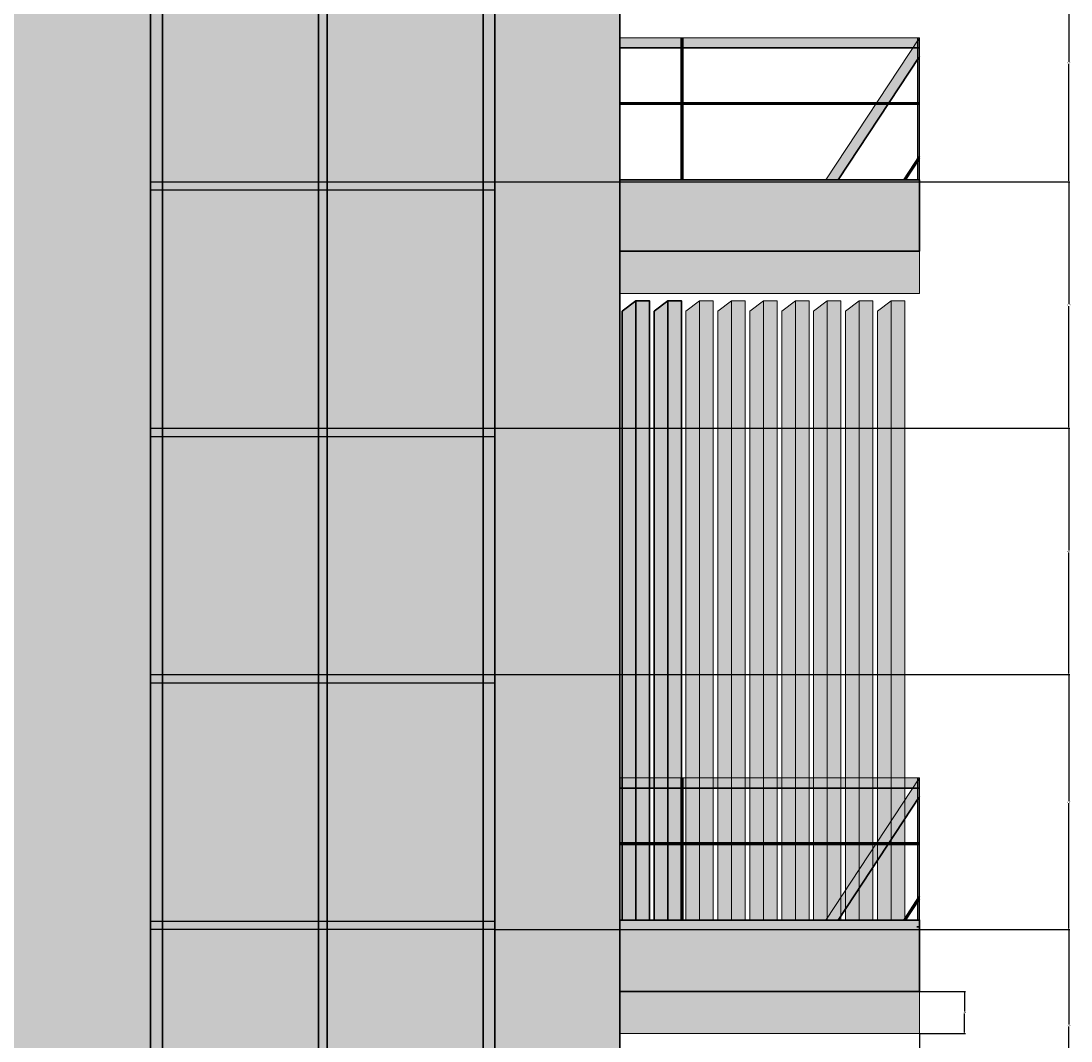
# Model space of a CAD drawing. Units: feet. Extents: x 2415 to 6174, y 866 to 1295.
# Tile 5 of 9: x 3580 to 3759, y 1010 to 1184. Entities that reach past the tile are written whole.
import ezdxf

# ---------------------------------------------------------------- set-up
doc = ezdxf.new("R2010")
doc.units = ezdxf.units.FT
for name, color, linetype, lineweight in [('A-ANNO-DIMS', 2, 'Continuous', 18), ('A-ELEV', 7, 'Continuous', 35), ('A-ELEV-LOUV', 9, 'Continuous', 18), ('A-ELEV-PATT', 8, 'Continuous', 13), ('A-ELEV-RAIL', 3, 'Continuous', 18), ('A-GLAZ', 4, 'Continuous', 25)]:
    doc.layers.add(name, color=color, linetype=linetype, lineweight=lineweight)
doc.styles.get("Standard").update_dxf_attribs({"font": 'arial.ttf'})
doc.dimstyles.get("Standard").update_dxf_attribs({"dimtxt": 0.18, "dimasz": 0.18, "dimexe": 0.18, "dimexo": 0.0625, "dimgap": 0.09, "dimtad": 0, "dimtih": 1, "dimtoh": 1, "dimdec": 1, "dimzin": 0, "dimdsep": 46, "dimlunit": 3, "dimtxsty": 'Standard', "dimcen": 0.09, "dimadec": 0, "dimazin": 0, "dimtfac": 1, "dimtdec": 1, "dimtofl": 0, "dimtmove": 0, "dimatfit": 3, "dimfxl": 1, "dimtolj": 1, "dimtzin": 0, "dimarcsym": 0})

# ---------------------------------------------------------------- blocks, each defined once
blk = doc.blocks.new('LOUVER-SLAT')
for p, q in [((2.33, 105.44), (0, 103.66)), ((0, 103.66), (0, 0))]:
    blk.add_line(p, q)
blk.add_lwpolyline([(2.33, 105.44), (4.65, 105.44), (4.65, 0), (2.33, 0)], close=True)
blk = doc.blocks.new('BALCONY-RAIL-PANEL')
for p, q in [((51.06, 33.86), (35.09, 9.65)), ((51.06, 0), (51.06, 33.86))]:
    blk.add_line(p, q)
for points in [[(0, 33.86), (51.06, 33.86)], [(50.67, 9.65), (50.67, 33.86)], [(51.06, 33.54), (50.91, 33.64)], [(50.93, 33.86), (50.93, 9.65)]]:
    blk.add_lwpolyline(points)
blk = doc.blocks.new('BALCONY-RAIL-BASE')
for p, q in [((51.06, 0), (51.06, 6)), ((0, 0), (51.06, 0))]:
    blk.add_line(p, q)
blk.add_lwpolyline([(51.06, 0), (0, 0), (0, 7.19), (51.06, 7.19)], close=True)
blk = doc.blocks.new('*D13')
at = {"layer": 'A-ANNO-DIMS', "color": 0, "lineweight": -2, "transparency": 16777216}
for p, q in [((3682.07, 1011.54), (3682.07, 1003.76)), ((3733.13, 1011.54), (3733.13, 1003.76)), ((3682.25, 1003.94), (3705.76, 1003.94)), ((3732.95, 1003.94), (3709.45, 1003.94))]:
    blk.add_line(p, q, dxfattribs=at)
at = {"layer": 'A-ANNO-DIMS', "color": 0, "transparency": 16777216}
for points in [[(3682.25, 1003.97), (3682.25, 1003.91), (3682.07, 1003.94)], [(3732.95, 1003.97), (3732.95, 1003.91), (3733.13, 1003.94)]]:
    blk.add_solid(points, dxfattribs=at)
at = {"layer": 'Defpoints', "color": 0, "transparency": 16777216}
for p in [(3682.07, 1011.6), (3733.13, 1011.6), (3733.13, 1003.94)]:
    blk.add_point(p, dxfattribs=at)
at = {"layer": 'A-ANNO-DIMS', "color": 0, "transparency": 16777216, "insert": (3707.6, 1003.94), "char_height": 0.18, "attachment_point": 5}
blk.add_mtext('\\A1;BALCONY RAIL BASE 51 TYP.', dxfattribs=at)
blk = doc.blocks.new('*D14')
at = {"layer": 'A-ANNO-DIMS', "color": 0, "lineweight": -2, "transparency": 16777216}
for p, q in [((3733.19, 1018.79), (3740.97, 1018.79)), ((3740.79, 1018.61), (3740.79, 1015.37)), ((3740.79, 1011.78), (3740.79, 1015.01)), ((3733.19, 1011.6), (3740.97, 1011.6))]:
    blk.add_line(p, q, dxfattribs=at)
at = {"layer": 'A-ANNO-DIMS', "color": 0, "transparency": 16777216}
for points in [[(3740.76, 1018.61), (3740.82, 1018.61), (3740.79, 1018.79)], [(3740.76, 1011.78), (3740.82, 1011.78), (3740.79, 1011.6)]]:
    blk.add_solid(points, dxfattribs=at)
at = {"layer": 'Defpoints', "color": 0, "transparency": 16777216}
for p in [(3733.13, 1018.79), (3740.79, 1018.79), (3733.13, 1011.6)]:
    blk.add_point(p, dxfattribs=at)
at = {"layer": 'A-ANNO-DIMS', "color": 0, "transparency": 16777216, "insert": (3740.79, 1015.19), "char_height": 0.18, "attachment_point": 5}
blk.add_mtext('\\A1;7 TYP.', dxfattribs=at)
blk = doc.blocks.new('*D82')
at = {"layer": 'A-ANNO-DIMS', "color": 0, "lineweight": -2, "transparency": 16777216}
for p, q in [((3660.88, 1029.3), (3758.71, 1029.3)), ((3758.53, 1029.12), (3758.53, 1013.16)), ((3758.53, 996.82), (3758.53, 1012.79)), ((3660.88, 996.64), (3758.71, 996.64))]:
    blk.add_line(p, q, dxfattribs=at)
at = {"layer": 'A-ANNO-DIMS', "color": 0, "transparency": 16777216}
for points in [[(3758.5, 1029.12), (3758.56, 1029.12), (3758.53, 1029.3)], [(3758.5, 996.82), (3758.56, 996.82), (3758.53, 996.64)]]:
    blk.add_solid(points, dxfattribs=at)
at = {"layer": 'Defpoints', "color": 0, "transparency": 16777216}
for p in [(3660.81, 1029.3), (3758.53, 1029.3), (3660.81, 996.64)]:
    blk.add_point(p, dxfattribs=at)
at = {"layer": 'A-ANNO-DIMS', "color": 0, "transparency": 16777216, "insert": (3758.53, 1012.97), "char_height": 0.18, "attachment_point": 5}
blk.add_mtext('\\A1;32.66', dxfattribs=at)
blk = doc.blocks.new('*D83')
at = {"layer": 'A-ANNO-DIMS', "color": 0, "lineweight": -2, "transparency": 16777216}
for p, q in [((3660.88, 1072.72), (3758.71, 1072.72)), ((3758.53, 1072.54), (3758.53, 1051.19)), ((3758.53, 1029.48), (3758.53, 1050.83)), ((3660.88, 1029.3), (3758.71, 1029.3))]:
    blk.add_line(p, q, dxfattribs=at)
at = {"layer": 'A-ANNO-DIMS', "color": 0, "transparency": 16777216}
for points in [[(3758.5, 1072.54), (3758.56, 1072.54), (3758.53, 1072.72)], [(3758.5, 1029.48), (3758.56, 1029.48), (3758.53, 1029.3)]]:
    blk.add_solid(points, dxfattribs=at)
at = {"layer": 'Defpoints', "color": 0, "transparency": 16777216}
for p in [(3660.81, 1072.72), (3758.53, 1072.72), (3660.81, 1029.3)]:
    blk.add_point(p, dxfattribs=at)
at = {"layer": 'A-ANNO-DIMS', "color": 0, "transparency": 16777216, "insert": (3758.53, 1051.01), "char_height": 0.18, "attachment_point": 5}
blk.add_mtext('\\A1;43.414', dxfattribs=at)
blk = doc.blocks.new('*D84')
at = {"layer": 'A-ANNO-DIMS', "color": 0, "lineweight": -2, "transparency": 16777216}
for p, q in [((3660.88, 1114.67), (3758.71, 1114.67)), ((3758.53, 1114.49), (3758.53, 1093.87)), ((3758.53, 1072.9), (3758.53, 1093.51)), ((3660.88, 1072.72), (3758.71, 1072.72))]:
    blk.add_line(p, q, dxfattribs=at)
at = {"layer": 'A-ANNO-DIMS', "color": 0, "transparency": 16777216}
for points in [[(3758.5, 1114.49), (3758.56, 1114.49), (3758.53, 1114.67)], [(3758.5, 1072.9), (3758.56, 1072.9), (3758.53, 1072.72)]]:
    blk.add_solid(points, dxfattribs=at)
at = {"layer": 'Defpoints', "color": 0, "transparency": 16777216}
for p in [(3660.81, 1114.67), (3758.53, 1114.67), (3660.81, 1072.72)]:
    blk.add_point(p, dxfattribs=at)
at = {"layer": 'A-ANNO-DIMS', "color": 0, "transparency": 16777216, "insert": (3758.53, 1093.69), "char_height": 0.18, "attachment_point": 5}
blk.add_mtext('\\A1;41.95', dxfattribs=at)
blk = doc.blocks.new('*D85')
at = {"layer": 'A-ANNO-DIMS', "color": 0, "lineweight": -2, "transparency": 16777216}
for p, q in [((3660.88, 1156.62), (3758.71, 1156.62)), ((3758.53, 1156.44), (3758.53, 1135.83)), ((3758.53, 1114.85), (3758.53, 1135.46)), ((3660.88, 1114.67), (3758.71, 1114.67))]:
    blk.add_line(p, q, dxfattribs=at)
at = {"layer": 'A-ANNO-DIMS', "color": 0, "transparency": 16777216}
for points in [[(3758.5, 1156.44), (3758.56, 1156.44), (3758.53, 1156.62)], [(3758.5, 1114.85), (3758.56, 1114.85), (3758.53, 1114.67)]]:
    blk.add_solid(points, dxfattribs=at)
at = {"layer": 'Defpoints', "color": 0, "transparency": 16777216}
for p in [(3660.81, 1156.62), (3758.53, 1156.62), (3660.81, 1114.67)]:
    blk.add_point(p, dxfattribs=at)
at = {"layer": 'A-ANNO-DIMS', "color": 0, "transparency": 16777216, "insert": (3758.53, 1135.65), "char_height": 0.18, "attachment_point": 5}
blk.add_mtext('\\A1;41.95', dxfattribs=at)
blk = doc.blocks.new('*D86')
at = {"layer": 'A-ANNO-DIMS', "color": 0, "lineweight": -2, "transparency": 16777216}
for p, q in [((3660.88, 1197.11), (3758.71, 1197.11)), ((3758.53, 1196.93), (3758.53, 1177.05)), ((3758.53, 1156.8), (3758.53, 1176.69)), ((3660.88, 1156.62), (3758.71, 1156.62))]:
    blk.add_line(p, q, dxfattribs=at)
at = {"layer": 'A-ANNO-DIMS', "color": 0, "transparency": 16777216}
for points in [[(3758.5, 1196.93), (3758.56, 1196.93), (3758.53, 1197.11)], [(3758.5, 1156.8), (3758.56, 1156.8), (3758.53, 1156.62)]]:
    blk.add_solid(points, dxfattribs=at)
at = {"layer": 'Defpoints', "color": 0, "transparency": 16777216}
for p in [(3660.81, 1197.11), (3758.53, 1197.11), (3660.81, 1156.62)]:
    blk.add_point(p, dxfattribs=at)
at = {"layer": 'A-ANNO-DIMS', "color": 0, "transparency": 16777216, "insert": (3758.53, 1176.87), "char_height": 0.18, "attachment_point": 5}
blk.add_mtext('\\A1;40.49', dxfattribs=at)

msp = doc.modelspace()

# ---------------------------------------------------------------- hatches: boundary and pattern name
at = {"layer": 'A-ELEV-PATT'}
h = msp.add_hatch(color=256, dxfattribs=at)
h.set_gradient(color1=(255, 255, 255), tint=1)
h.paths.add_polyline_path([(3264.916, 1143.5993), (3253.129, 1143.5993), (3253.129, 891.5993), (3264.916, 891.5993)])
h.paths.add_polyline_path([(3470.0448, 1143.5993), (3264.916, 1143.5993), (3264.916, 1137.5993), (3466.5999, 1137.5993)])
h.paths.add_polyline_path([(3363.8667, 1137.5993), (3264.916, 1137.5993), (3264.916, 1011.5993), (3363.8667, 1011.5993)])
h.paths.add_polyline_path([(3286.0429, 1117.0591), (3337.7904, 1117.0591), (3337.7904, 1115.4381), (3336.5314, 1115.4381), (3336.5314, 1110.528), (3335.4882, 1110.528), (3335.4882, 1042.3194), (3288.3452, 1042.3194), (3288.3452, 1110.528), (3287.3019, 1110.528), (3287.3019, 1115.4381), (3286.0429, 1115.4381)], flags=16)
h.paths.add_polyline_path([(3290.3452, 1108.528), (3333.4882, 1108.528), (3333.4882, 1044.3194), (3290.3452, 1044.3194)], flags=0)
h.paths.add_polyline_path([(3292.3452, 1106.528), (3331.4882, 1106.528), (3331.4882, 1046.3194), (3292.3452, 1046.3194)], flags=0)
h.paths.add_polyline_path([(3311.7156, 1106.528), (3312.1178, 1106.528), (3312.1178, 1046.3194), (3311.7156, 1046.3194)], flags=0)
h.paths.add_polyline_path([(3682.0722, 1263.5993), (3578.5579, 1263.5993), (3578.5579, 1137.5993), (3578.5579, 961.3655), (3682.0722, 961.3655)])
h.paths.add_polyline_path([(3660.8129, 1239.0671), (3660.8129, 996.6447), (3602.2151, 996.6447), (3602.2151, 1239.0671)], flags=16)
h.paths.add_polyline_path([(3632.2447, 1239.0671), (3632.2447, 996.6447), (3630.7833, 996.6447), (3630.7833, 1029.3019), (3602.2151, 1029.3019), (3602.2151, 1030.7632), (3630.7833, 1030.7632), (3630.7833, 1071.2549), (3602.2151, 1071.2549), (3602.2151, 1072.7163), (3630.7833, 1072.7163), (3630.7833, 1113.2079), (3602.2151, 1113.2079), (3602.2151, 1114.6693), (3630.7833, 1114.6693), (3630.7833, 1155.161), (3602.2151, 1155.161), (3602.2151, 1156.6224), (3630.7833, 1156.6224), (3630.7833, 1197.114), (3602.2151, 1197.114), (3602.2151, 1198.5754), (3630.7833, 1198.5754), (3630.7833, 1239.0671)], flags=0)
h.paths.add_polyline_path([(3733.129, 951.5993), (3634.5374, 951.5993), (3634.5374, 891.5993), (3733.129, 891.5993)])
h.paths.add_polyline_path([(3627.8799, 951.5993), (3621.0953, 951.5993), (3621.0953, 891.5993), (3627.8799, 891.5993)])
h.paths.add_polyline_path([(3614.4378, 951.5993), (3607.6532, 951.5993), (3607.6532, 891.5993), (3614.4378, 891.5993)])
h.paths.add_polyline_path([(3565.9347, 951.5993), (3441.3079, 951.5993), (3441.3079, 891.5993), (3565.9347, 891.5993)], flags=17)
h.paths.add_polyline_path([(3571.9347, 957.5993), (3435.3079, 957.5993), (3435.3079, 891.5993), (3441.3079, 891.5993), (3441.3079, 951.5993), (3565.9347, 951.5993), (3565.9347, 891.5993), (3571.9347, 891.5993)])
h.paths.add_polyline_path([(3435.3079, 1011.5993), (3423.5209, 1011.5993), (3423.5209, 891.5993), (3435.3079, 891.5993), (3435.3079, 957.5993)])
h.paths.add_polyline_path([(3690.0912, 1269.5993), (3571.9347, 1269.5993), (3571.9347, 1263.5993), (3690.0912, 1263.5993)])
h.paths.add_polyline_path([(3571.9347, 1269.5993), (3538.5122, 1257.6449), (3538.5122, 1251.6449), (3571.9347, 1263.5993)])
h = msp.add_hatch(color=256, dxfattribs=at)
h.set_gradient(color1=(99, 100, 102), color2=(99, 100, 102))
h.paths.add_polyline_path([(3660.8129, 1239.0671), (3602.2151, 1239.0671), (3602.2151, 996.6447), (3660.8129, 996.6447)])
h.paths.add_polyline_path([(3604.2151, 1237.0671), (3658.8129, 1237.0671), (3658.8129, 998.6447), (3604.2151, 998.6447)], flags=16)
h = msp.add_hatch(color=256, dxfattribs=at)
h.set_gradient(color1=(181, 210, 237), color2=(122, 175, 223))
h.paths.add_polyline_path([(3630.7833, 1239.0671), (3602.2151, 1239.0671), (3602.2151, 1198.5754), (3630.7833, 1198.5754)])
h.paths.add_polyline_path([(3660.8129, 1239.0671), (3632.2447, 1239.0671), (3632.2447, 1198.5754), (3660.8129, 1198.5754)])
h.paths.add_polyline_path([(3630.7833, 1197.114), (3602.2151, 1197.114), (3602.2151, 1156.6224), (3630.7833, 1156.6224)])
h.paths.add_polyline_path([(3660.8129, 1197.114), (3632.2447, 1197.114), (3632.2447, 1156.6224), (3660.8129, 1156.6224)])
h.paths.add_polyline_path([(3630.7833, 1155.161), (3602.2151, 1155.161), (3602.2151, 1114.6693), (3630.7833, 1114.6693)])
h.paths.add_polyline_path([(3660.8129, 1155.161), (3632.2447, 1155.161), (3632.2447, 1114.6693), (3660.8129, 1114.6693)])
h.paths.add_polyline_path([(3630.7833, 1113.2079), (3602.2151, 1113.2079), (3602.2151, 1072.7163), (3630.7833, 1072.7163)])
h.paths.add_polyline_path([(3660.8129, 1113.2079), (3632.2447, 1113.2079), (3632.2447, 1072.7163), (3660.8129, 1072.7163)])
h.paths.add_polyline_path([(3660.8129, 1071.2549), (3632.2447, 1071.2549), (3632.2447, 996.6447), (3660.8129, 996.6447)])
h.paths.add_polyline_path([(3630.7833, 1071.2549), (3602.2151, 1071.2549), (3602.2151, 1030.7632), (3630.7833, 1030.7632)])
h.paths.add_polyline_path([(3630.7833, 1029.3019), (3602.2151, 1029.3019), (3602.2151, 996.6447), (3630.7833, 996.6447)])
h = msp.add_hatch(color=256, dxfattribs=at)
h.set_gradient(color2=(0, 0, 0))
h.paths.add_polyline_path([(3630.7833, 1030.7632), (3604.2151, 1030.7632), (3604.2151, 1029.3019), (3630.7833, 1029.3019)])
h.paths.add_polyline_path([(3658.8129, 1030.7632), (3632.2447, 1030.7632), (3632.2447, 1029.3019), (3658.8129, 1029.3019)])
h.paths.add_polyline_path([(3632.2447, 1030.7632), (3630.7833, 1030.7632), (3630.7833, 1029.3019), (3632.2447, 1029.3019)])
h.paths.add_polyline_path([(3632.2447, 1239.0671), (3630.7833, 1239.0671), (3630.7833, 1030.7632), (3632.2447, 1030.7632)])
h.paths.add_polyline_path([(3632.2447, 1029.3019), (3630.7833, 1029.3019), (3630.7833, 996.6447), (3632.2447, 996.6447)])
h = msp.add_hatch(color=256, dxfattribs=at)
h.set_gradient(color1=(205, 105, 40), color2=(205, 105, 40))
h.paths.add_polyline_path([(3578.5579, 1203.5993), (3509.1068, 1203.5993), (3471.2123, 1137.5993), (3578.5579, 1137.5993)])
h.paths.add_polyline_path([(3521.9379, 1169.0289), (3521.9379, 1158.6726), (3512.0517, 1158.6726), (3512.0517, 1169.0289)], flags=16)
h.paths.add_polyline_path([(3534.3754, 1169.0289), (3544.2616, 1169.0289), (3544.2616, 1158.6726), (3534.3754, 1158.6726)], flags=16)
h.paths.add_polyline_path([(3556.6991, 1169.0289), (3566.5853, 1169.0289), (3566.5853, 1158.6726), (3556.6991, 1158.6726)], flags=16)
h.paths.add_polyline_path([(3687.1301, 1136.3701), (3684.8039, 1136.3701), (3684.8039, 1030.9315), (3687.1301, 1030.9315)])
h.paths.add_polyline_path([(3692.5646, 1136.3701), (3690.2384, 1136.3701), (3690.2384, 1030.9315), (3692.5646, 1030.9315)])
h.paths.add_polyline_path([(3697.9991, 1136.3701), (3695.6729, 1136.3701), (3695.6729, 1030.9315), (3697.9991, 1030.9315)])
h.paths.add_polyline_path([(3703.4336, 1136.3701), (3701.1074, 1136.3701), (3701.1074, 1030.9315), (3703.4336, 1030.9315)])
h.paths.add_polyline_path([(3708.8681, 1136.3701), (3706.5419, 1136.3701), (3706.5419, 1030.9315), (3708.8681, 1030.9315)])
h.paths.add_polyline_path([(3714.3026, 1136.3701), (3711.9764, 1136.3701), (3711.9764, 1030.9315), (3714.3026, 1030.9315)])
h.paths.add_polyline_path([(3719.7371, 1136.3701), (3717.4109, 1136.3701), (3717.4109, 1030.9315), (3719.7371, 1030.9315)])
h.paths.add_polyline_path([(3725.1716, 1136.3701), (3722.8454, 1136.3701), (3722.8454, 1030.9315), (3725.1716, 1030.9315)])
h.paths.add_polyline_path([(3730.6061, 1136.3701), (3728.2799, 1136.3701), (3728.2799, 1030.9315), (3730.6061, 1030.9315)])
h.paths.add_polyline_path([(3382.3104, 1123.5993), (3377.658, 1123.5993), (3377.658, 1053.4585), (3382.3104, 1053.4585)], flags=17)
h.paths.add_polyline_path([(3390.153, 1123.5993), (3385.5006, 1123.5993), (3385.5006, 1053.4585), (3390.153, 1053.4585)], flags=17)
h.paths.add_polyline_path([(3382.3104, 1129.5993), (3377.658, 1129.5993), (3377.658, 1123.5993), (3382.3104, 1123.5993)], flags=17)
h.paths.add_polyline_path([(3390.153, 1129.5993), (3385.5006, 1129.5993), (3385.5006, 1123.5993), (3390.153, 1123.5993)], flags=17)
h.paths.add_polyline_path([(3397.9956, 1129.5993), (3393.3432, 1129.5993), (3393.3432, 1123.5993), (3397.9956, 1123.5993)])
h.paths.add_polyline_path([(3397.9956, 1123.5993), (3393.3432, 1123.5993), (3393.3432, 1019.5993), (3397.9956, 1019.5993)])
h.paths.add_polyline_path([(3405.8382, 1129.5993), (3401.1858, 1129.5993), (3401.1858, 1123.5993), (3405.8382, 1123.5993)])
h.paths.add_polyline_path([(3405.8382, 1123.5993), (3401.1858, 1123.5993), (3401.1858, 1019.5993), (3405.8382, 1019.5993)])
h.paths.add_polyline_path([(3413.6808, 1129.5993), (3409.0284, 1129.5993), (3409.0284, 1123.5993), (3413.6808, 1123.5993)])
h.paths.add_polyline_path([(3413.6808, 1123.5993), (3409.0284, 1123.5993), (3409.0284, 1019.5993), (3413.6808, 1019.5993)])
h.paths.add_polyline_path([(3421.5234, 1129.5993), (3416.871, 1129.5993), (3416.871, 1123.5993), (3421.5234, 1123.5993)])
h.paths.add_polyline_path([(3421.5234, 1123.5993), (3416.871, 1123.5993), (3416.871, 1019.5993), (3421.5234, 1019.5993)])
h.paths.add_polyline_path([(3429.366, 1129.5993), (3424.7136, 1129.5993), (3424.7136, 1123.5993), (3429.366, 1123.5993)])
h.paths.add_polyline_path([(3429.366, 1123.5993), (3424.7136, 1123.5993), (3424.7136, 1019.5993), (3429.366, 1019.5993)])
h.paths.add_polyline_path([(3437.2086, 1129.5993), (3432.5562, 1129.5993), (3432.5562, 1123.5993), (3437.2086, 1123.5993)])
h.paths.add_polyline_path([(3437.2086, 1123.5993), (3432.5562, 1123.5993), (3432.5562, 1019.5993), (3437.2086, 1019.5993)])
h.paths.add_polyline_path([(3446.1534, 1129.5993), (3440.3202, 1129.5993), (3440.3202, 1123.5993), (3446.1534, 1123.5993)])
h.paths.add_polyline_path([(3446.1534, 1123.5993), (3440.3202, 1123.5993), (3440.3202, 1019.5993), (3446.1534, 1019.5993)])
h.paths.add_polyline_path([(3390.153, 1123.5993), (3385.5006, 1123.5993), (3385.5006, 1053.4585), (3385.5006, 1019.5993), (3390.153, 1019.5993)])
h.paths.add_polyline_path([(3390.153, 1123.5993), (3390.153, 1129.5993), (3385.5006, 1129.5993), (3385.5006, 1053.4585), (3390.153, 1053.4585)])
h.paths.add_polyline_path([(3382.3104, 1027.963), (3377.658, 1027.963), (3377.658, 1019.5993), (3382.3104, 1019.5993)])
h.paths.add_polyline_path([(3382.3104, 1028.2269), (3377.658, 1028.2269), (3377.658, 1027.963), (3382.3104, 1027.963)])
h.paths.add_polyline_path([(3382.3104, 1129.5993), (3377.658, 1129.5993), (3377.658, 1028.2269), (3382.3104, 1028.2269)])
h = msp.add_hatch(color=256, dxfattribs=at)
h.set_gradient(color2=(0, 0, 0))
h.paths.add_polyline_path([(3489.4854, 1177.4585), (3454.5146, 1177.4585), (3454.5146, 1175.7117), (3488.4825, 1175.7117)])
h.paths.add_polyline_path([(3454.5146, 1177.4585), (3454.2507, 1177.4585), (3454.2507, 1175.7117), (3454.5146, 1175.7117)])
h.paths.add_polyline_path([(3454.5146, 1175.7117), (3454.2507, 1175.7117), (3454.2507, 1166.3873), (3454.5146, 1166.3873)])
h.paths.add_polyline_path([(3454.5146, 1166.3873), (3454.2507, 1166.3873), (3454.2507, 1166.1234), (3454.5146, 1166.1234)])
h.paths.add_polyline_path([(3483.1288, 1166.3873), (3454.5146, 1166.3873), (3454.5146, 1166.1234), (3482.9773, 1166.1234)])
h.paths.add_polyline_path([(3454.2507, 1166.3873), (3414.3148, 1166.3873), (3414.3148, 1166.1234), (3454.2507, 1166.1234)])
h.paths.add_polyline_path([(3454.5146, 1166.1234), (3454.2507, 1166.1234), (3454.2507, 1152.2269), (3454.5146, 1152.2269)])
h.paths.add_polyline_path([(3454.5146, 1152.2269), (3454.2507, 1152.2269), (3454.2507, 1151.963), (3454.5146, 1151.963)])
h.paths.add_polyline_path([(3474.9985, 1152.2269), (3454.5146, 1152.2269), (3454.5146, 1151.963), (3474.8469, 1151.963)])
h.paths.add_polyline_path([(3454.2507, 1152.2269), (3414.3148, 1152.2269), (3414.3148, 1151.963), (3454.2507, 1151.963)])
h.paths.add_polyline_path([(3454.5146, 1151.963), (3454.2507, 1151.963), (3454.2507, 1143.5993), (3454.5146, 1143.5993)])
h.paths.add_polyline_path([(3414.3148, 1175.7117), (3414.0509, 1175.7117), (3414.0509, 1166.3873), (3414.3148, 1166.3873)])
h.paths.add_polyline_path([(3414.3148, 1166.1234), (3414.0509, 1166.1234), (3414.0509, 1152.2269), (3414.3148, 1152.2269)])
h.paths.add_polyline_path([(3414.3148, 1152.2269), (3414.0509, 1152.2269), (3414.0509, 1151.963), (3414.3148, 1151.963)])
h.paths.add_polyline_path([(3414.3148, 1151.963), (3414.0509, 1151.963), (3414.0509, 1143.5993), (3414.3148, 1143.5993)])
h.paths.add_polyline_path([(3414.0509, 1152.2269), (3374.115, 1152.2269), (3374.115, 1151.963), (3414.0509, 1151.963)])
h.paths.add_polyline_path([(3374.115, 1166.1234), (3373.851, 1166.1234), (3373.851, 1152.2269), (3374.115, 1152.2269)])
h.paths.add_polyline_path([(3374.115, 1151.963), (3373.851, 1151.963), (3373.851, 1143.5993), (3374.115, 1143.5993)])
h.paths.add_polyline_path([(3363.6028, 1172.4585), (3333.9151, 1172.4585), (3333.9151, 1170.7117), (3363.6028, 1170.7117)])
h.paths.add_polyline_path([(3293.4514, 1172.4585), (3253.5155, 1172.4585), (3253.5155, 1171.8725), (3254.2811, 1170.7117), (3293.4514, 1170.7117)])
h.paths.add_polyline_path([(3333.6512, 1172.4585), (3293.7153, 1172.4585), (3293.7153, 1170.7117), (3333.6512, 1170.7117)])
h.paths.add_polyline_path([(3293.7153, 1172.4585), (3293.4514, 1172.4585), (3293.4514, 1170.7117), (3293.7153, 1170.7117)])
h.paths.add_polyline_path([(3333.9151, 1172.4585), (3333.6512, 1172.4585), (3333.6512, 1170.7117), (3333.9151, 1170.7117)])
h.paths.add_polyline_path([(3333.9151, 1170.7117), (3333.6512, 1170.7117), (3333.6512, 1161.3873), (3333.9151, 1161.3873)])
h.paths.add_polyline_path([(3333.9151, 1161.3873), (3333.6512, 1161.3873), (3333.6512, 1161.1234), (3333.9151, 1161.1234)])
h.paths.add_polyline_path([(3363.6028, 1161.3873), (3333.9151, 1161.3873), (3333.9151, 1161.1234), (3363.6028, 1161.1234)])
h.paths.add_polyline_path([(3333.6512, 1161.3873), (3293.7153, 1161.3873), (3293.7153, 1161.1234), (3333.6512, 1161.1234)])
h.paths.add_polyline_path([(3333.9151, 1161.1234), (3333.6512, 1161.1234), (3333.6512, 1147.2269), (3333.9151, 1147.2269)])
h.paths.add_polyline_path([(3333.9151, 1147.2269), (3333.6512, 1147.2269), (3333.6512, 1146.963), (3333.9151, 1146.963)])
h.paths.add_polyline_path([(3333.9151, 1146.963), (3333.6512, 1146.963), (3333.6512, 1143.5993), (3333.9151, 1143.5993)])
h.paths.add_polyline_path([(3363.6028, 1147.2269), (3333.9151, 1147.2269), (3333.9151, 1146.963), (3363.6028, 1146.963)])
h.paths.add_polyline_path([(3333.6512, 1147.2269), (3293.7153, 1147.2269), (3293.7153, 1146.963), (3333.6512, 1146.963)])
h.paths.add_polyline_path([(3293.7153, 1170.7117), (3293.4514, 1170.7117), (3293.4514, 1161.3873), (3293.7153, 1161.3873)])
h.paths.add_polyline_path([(3293.7153, 1161.1234), (3293.4514, 1161.1234), (3293.4514, 1147.2269), (3293.7153, 1147.2269)])
h.paths.add_polyline_path([(3293.7153, 1161.3873), (3293.4514, 1161.3873), (3293.4514, 1161.1234), (3293.7153, 1161.1234)])
h.paths.add_polyline_path([(3293.4514, 1161.3873), (3260.4316, 1161.3873), (3260.6056, 1161.1234), (3293.4514, 1161.1234)])
h.paths.add_polyline_path([(3293.7153, 1147.2269), (3293.4514, 1147.2269), (3293.4514, 1146.963), (3293.7153, 1146.963)])
h.paths.add_polyline_path([(3293.7153, 1146.963), (3293.4514, 1146.963), (3293.4514, 1143.5993), (3293.7153, 1143.5993)])
h.paths.add_polyline_path([(3293.4514, 1147.2269), (3269.7719, 1147.2269), (3269.946, 1146.963), (3293.4514, 1146.963)])
h.paths.add_polyline_path([(3254.2811, 1170.7117), (3253.5155, 1170.7117), (3253.5155, 1168.7002), (3258.3391, 1161.3873), (3260.4316, 1161.3873)])
h.paths.add_polyline_path([(3260.4316, 1161.3873), (3258.3391, 1161.3873), (3258.5131, 1161.1234), (3260.6056, 1161.1234)])
h.paths.add_polyline_path([(3260.6056, 1161.1234), (3258.5131, 1161.1234), (3267.6794, 1147.2269), (3269.7719, 1147.2269)])
h.paths.add_polyline_path([(3258.3391, 1161.3873), (3253.5155, 1161.3873), (3253.5155, 1161.1234), (3258.5131, 1161.1234)])
h.paths.add_polyline_path([(3269.7719, 1147.2269), (3267.6794, 1147.2269), (3267.8535, 1146.963), (3269.946, 1146.963)])
h.paths.add_polyline_path([(3269.946, 1146.963), (3267.8535, 1146.963), (3270.0722, 1143.5993), (3272.1647, 1143.5993)])
h.paths.add_polyline_path([(3267.6794, 1147.2269), (3256.5092, 1147.2269), (3256.6833, 1146.963), (3267.8535, 1146.963)])
h.paths.add_polyline_path([(3256.1931, 1147.2269), (3253.5155, 1147.2269), (3253.5155, 1146.963), (3256.3671, 1146.963)])
h.paths.add_polyline_path([(3253.5155, 1151.7656), (3253.5155, 1151.2863), (3256.1931, 1147.2269), (3256.5092, 1147.2269)])
h.paths.add_polyline_path([(3256.5092, 1147.2269), (3256.1931, 1147.2269), (3256.3671, 1146.963), (3256.6833, 1146.963)])
h.paths.add_polyline_path([(3256.6833, 1146.963), (3256.3671, 1146.963), (3258.5859, 1143.5993), (3258.902, 1143.5993)])
h.paths.add_polyline_path([(3253.2515, 1152.1657), (3253.2515, 1151.6864), (3253.5155, 1151.2863), (3253.5155, 1151.7656)])
h.paths.add_polyline_path([(3253.5155, 1168.7002), (3253.2515, 1169.1003), (3253.2515, 1152.1657), (3253.5155, 1151.7656)])
h.paths.add_polyline_path([(3253.5155, 1151.2863), (3253.2515, 1151.6864), (3253.2515, 1147.2269), (3253.5155, 1147.2269)])
h.paths.add_polyline_path([(3253.5155, 1147.2269), (3253.2515, 1147.2269), (3253.2515, 1146.963), (3253.5155, 1146.963)])
h.paths.add_polyline_path([(3253.5155, 1146.963), (3253.2515, 1146.963), (3253.2515, 1143.5993), (3253.5155, 1143.5993)])
h.paths.add_polyline_path([(3253.5155, 1171.8725), (3253.2515, 1172.2726), (3253.2515, 1169.1003), (3253.5155, 1168.7002)])
h.paths.add_polyline_path([(3253.5155, 1172.4585), (3253.2515, 1172.4585), (3253.2515, 1172.2726), (3253.5155, 1171.8725)])
h.paths.add_polyline_path([(3253.5155, 1171.8725), (3253.5155, 1170.7117), (3254.2811, 1170.7117)], flags=17)
h.paths.add_polyline_path([(3692.5426, 1181.1411), (3682.0722, 1181.1411), (3682.0722, 1179.3943), (3692.5426, 1179.3943)])
h.paths.add_polyline_path([(3732.7425, 1180.5551), (3732.7425, 1181.1411), (3692.8065, 1181.1411), (3692.8065, 1179.3943), (3731.9768, 1179.3943)])
h.paths.add_polyline_path([(3692.8065, 1181.1411), (3692.5426, 1181.1411), (3692.5426, 1179.3943), (3692.8065, 1179.3943)])
h.paths.add_polyline_path([(3692.8065, 1179.3943), (3692.5426, 1179.3943), (3692.5426, 1170.0699), (3692.8065, 1170.0699)])
h.paths.add_polyline_path([(3725.8264, 1170.0699), (3692.8065, 1170.0699), (3692.8065, 1169.806), (3725.6523, 1169.806)])
h.paths.add_polyline_path([(3692.5426, 1170.0699), (3682.0722, 1170.0699), (3682.0722, 1169.806), (3692.5426, 1169.806)])
h.paths.add_polyline_path([(3692.8065, 1170.0699), (3692.5426, 1170.0699), (3692.5426, 1169.806), (3692.8065, 1169.806)])
h.paths.add_polyline_path([(3692.8065, 1169.806), (3692.5426, 1169.806), (3692.5426, 1156.9315), (3692.8065, 1156.9315)])
h.paths.add_polyline_path([(3733.0064, 1180.9552), (3733.0064, 1181.1411), (3732.7425, 1181.1411), (3732.7425, 1180.5551)])
h.paths.add_polyline_path([(3733.0064, 1180.9058), (3732.9836, 1180.9208), (3732.7425, 1180.5551), (3732.7425, 1179.3943), (3733.0064, 1179.3943)])
h.paths.add_polyline_path([(3732.7425, 1180.5551), (3731.9768, 1179.3943), (3732.7425, 1179.3943)], flags=17)
h.paths.add_polyline_path([(3732.7425, 1179.3943), (3731.9768, 1179.3943), (3725.8264, 1170.0699), (3727.9189, 1170.0699), (3732.7425, 1177.3828)])
h.paths.add_polyline_path([(3733.0064, 1179.3943), (3732.7425, 1179.3943), (3732.7425, 1177.3828), (3733.0064, 1177.7829)])
h.paths.add_polyline_path([(3733.0064, 1170.0699), (3732.7425, 1170.0699), (3732.7425, 1169.806), (3733.0064, 1169.806)])
h.paths.add_polyline_path([(3733.0064, 1177.7829), (3732.7425, 1177.3828), (3732.7425, 1170.0699), (3733.0064, 1170.0699)])
h.paths.add_polyline_path([(3732.7425, 1170.0699), (3727.9189, 1170.0699), (3727.7448, 1169.806), (3732.7425, 1169.806)])
h.paths.add_polyline_path([(3727.9189, 1170.0699), (3725.8264, 1170.0699), (3725.6523, 1169.806), (3727.7448, 1169.806)])
h.paths.add_polyline_path([(3727.7448, 1169.806), (3725.6523, 1169.806), (3717.1602, 1156.9315), (3719.2527, 1156.9315)])
h.paths.add_polyline_path([(3733.0064, 1160.369), (3733.0064, 1160.8483), (3732.7425, 1160.4482), (3732.7425, 1159.9689)])
h.paths.add_polyline_path([(3733.0064, 1169.806), (3732.7425, 1169.806), (3732.7425, 1160.4482), (3733.0064, 1160.8483)])
h.paths.add_polyline_path([(3733.0064, 1160.369), (3732.7425, 1159.9689), (3732.7425, 1156.9315), (3733.0064, 1156.9315)])
h = msp.add_hatch(color=256, dxfattribs=at)
h.set_gradient(color2=(0, 0, 0))
h.paths.add_polyline_path([(3630.7833, 1156.6224), (3604.2151, 1156.6224), (3604.2151, 1155.161), (3630.7833, 1155.161)])
h.paths.add_polyline_path([(3658.8129, 1156.6224), (3632.2447, 1156.6224), (3632.2447, 1155.161), (3658.8129, 1155.161)])
h = msp.add_hatch(color=256, dxfattribs=at)
h.set_gradient(color1=(99, 100, 102), color2=(99, 100, 102))
h.paths.add_polyline_path([(3733.129, 1156.9315), (3682.0722, 1156.9315), (3682.0722, 1144.7857), (3733.129, 1144.7857)])
h.paths.add_polyline_path([(3733.129, 1144.7857), (3682.0722, 1144.7857), (3682.0722, 1137.5993), (3733.129, 1137.5993)])
h.paths.add_polyline_path([(3733.129, 1018.7857), (3682.0722, 1018.7857), (3682.0722, 1011.5993), (3733.129, 1011.5993)])
h.paths.add_polyline_path([(3733.129, 1030.9315), (3682.0722, 1030.9315), (3682.0722, 1018.7857), (3733.129, 1018.7857)])
h = msp.add_hatch(color=256, dxfattribs=at)
h.set_gradient(color1=(208, 121, 6), color2=(208, 121, 6))
h.paths.add_polyline_path([(3684.8039, 1136.3701), (3682.4777, 1134.5952), (3682.4777, 1030.9315), (3684.8039, 1030.9315)])
h = msp.add_hatch(color=256, dxfattribs=at)
h.set_gradient(color1=(208, 121, 6), color2=(208, 121, 6))
h.paths.add_polyline_path([(3690.2384, 1136.3701), (3687.9122, 1134.5952), (3687.9122, 1030.9315), (3690.2384, 1030.9315)])
h = msp.add_hatch(color=256, dxfattribs=at)
h.set_gradient(color1=(208, 121, 6), color2=(208, 121, 6))
h.paths.add_polyline_path([(3695.6729, 1136.3701), (3693.3467, 1134.5952), (3693.3467, 1030.9315), (3695.6729, 1030.9315)])
h = msp.add_hatch(color=256, dxfattribs=at)
h.set_gradient(color1=(208, 121, 6), color2=(208, 121, 6))
h.paths.add_polyline_path([(3701.1074, 1136.3701), (3698.7812, 1134.5952), (3698.7812, 1030.9315), (3701.1074, 1030.9315)])
h = msp.add_hatch(color=256, dxfattribs=at)
h.set_gradient(color1=(208, 121, 6), color2=(208, 121, 6))
h.paths.add_polyline_path([(3706.5419, 1136.3701), (3704.2157, 1134.5952), (3704.2157, 1030.9315), (3706.5419, 1030.9315)])
h = msp.add_hatch(color=256, dxfattribs=at)
h.set_gradient(color1=(208, 121, 6), color2=(208, 121, 6))
h.paths.add_polyline_path([(3711.9764, 1136.3701), (3709.6502, 1134.5952), (3709.6502, 1030.9315), (3711.9764, 1030.9315)])
h = msp.add_hatch(color=256, dxfattribs=at)
h.set_gradient(color1=(208, 121, 6), color2=(208, 121, 6))
h.paths.add_polyline_path([(3717.4109, 1136.3701), (3715.0847, 1134.5952), (3715.0847, 1030.9315), (3717.4109, 1030.9315)])
h = msp.add_hatch(color=256, dxfattribs=at)
h.set_gradient(color1=(208, 121, 6), color2=(208, 121, 6))
h.paths.add_polyline_path([(3722.8454, 1136.3701), (3720.5192, 1134.5952), (3720.5192, 1030.9315), (3722.8454, 1030.9315)])
h = msp.add_hatch(color=256, dxfattribs=at)
h.set_gradient(color1=(208, 121, 6), color2=(208, 121, 6))
h.paths.add_polyline_path([(3728.2799, 1136.3701), (3725.9537, 1134.5952), (3725.9537, 1030.9315), (3728.2799, 1030.9315)])
h = msp.add_hatch(color=256, dxfattribs=at)
h.set_gradient(color2=(0, 0, 0))
h.paths.add_polyline_path([(3630.7833, 1114.6693), (3604.2151, 1114.6693), (3604.2151, 1113.2079), (3630.7833, 1113.2079)])
h.paths.add_polyline_path([(3658.8129, 1114.6693), (3632.2447, 1114.6693), (3632.2447, 1113.2079), (3658.8129, 1113.2079)])
h = msp.add_hatch(color=256, dxfattribs=at)
h.set_gradient(color2=(0, 0, 0))
h.paths.add_polyline_path([(3630.7833, 1072.7163), (3604.2151, 1072.7163), (3604.2151, 1071.2549), (3630.7833, 1071.2549)])
h.paths.add_polyline_path([(3658.8129, 1072.7163), (3632.2447, 1072.7163), (3632.2447, 1071.2549), (3658.8129, 1071.2549)])
h = msp.add_hatch(color=256, dxfattribs=at)
h.set_gradient(color2=(0, 0, 0))
h.paths.add_polyline_path([(3684.8039, 1055.1411), (3682.4777, 1055.1411), (3682.4777, 1053.3943), (3684.8039, 1053.3943)])
h.paths.add_polyline_path([(3682.4777, 1055.1411), (3682.0722, 1055.1411), (3682.0722, 1053.3943), (3682.4777, 1053.3943)])
h.paths.add_polyline_path([(3687.1301, 1055.1411), (3684.8039, 1055.1411), (3684.8039, 1053.3943), (3687.1301, 1053.3943)])
h.paths.add_polyline_path([(3687.9122, 1055.1411), (3687.1301, 1055.1411), (3687.1301, 1053.3943), (3687.9122, 1053.3943)])
h.paths.add_polyline_path([(3690.2384, 1055.1411), (3687.9122, 1055.1411), (3687.9122, 1053.3943), (3690.2384, 1053.3943)])
h.paths.add_polyline_path([(3692.5426, 1055.1411), (3690.2384, 1055.1411), (3690.2384, 1053.3943), (3692.5426, 1053.3943)])
h = msp.add_hatch(color=256, dxfattribs=at)
h.set_gradient(color2=(0, 0, 0))
h.paths.add_polyline_path([(3692.5426, 1055.1411), (3682.0722, 1055.1411), (3682.0722, 1053.3943), (3692.5426, 1053.3943)])
h.paths.add_polyline_path([(3732.7425, 1054.5551), (3732.7425, 1055.1411), (3692.8065, 1055.1411), (3692.8065, 1053.3943), (3731.9768, 1053.3943)])
h.paths.add_polyline_path([(3692.8065, 1055.1411), (3692.5426, 1055.1411), (3692.5426, 1053.3943), (3692.8065, 1053.3943)])
h.paths.add_polyline_path([(3733.0064, 1054.9552), (3733.0064, 1055.1411), (3732.7425, 1055.1411), (3732.7425, 1054.5551)])
h.paths.add_polyline_path([(3733.0064, 1054.9058), (3732.9836, 1054.9208), (3732.7425, 1054.5551), (3732.7425, 1053.3943), (3733.0064, 1053.3943)])
h.paths.add_polyline_path([(3733.129, 1055.1411), (3733.0064, 1055.1411), (3733.0064, 1054.9552)], flags=17)
h.paths.add_polyline_path([(3733.129, 1055.1411), (3733.0064, 1054.9552), (3733.0064, 1054.9058), (3733.129, 1054.8249)])
h.paths.add_polyline_path([(3733.0064, 1054.9552), (3732.9836, 1054.9208), (3733.0064, 1054.9058)], flags=17)
h.paths.add_polyline_path([(3733.129, 1054.8249), (3733.0064, 1054.9058), (3733.0064, 1053.3943), (3733.129, 1053.3943)])
h.paths.add_polyline_path([(3732.7425, 1054.5551), (3731.9768, 1053.3943), (3732.7425, 1053.3943)], flags=17)
h.paths.add_polyline_path([(3732.7425, 1051.3828), (3732.7425, 1053.3943), (3731.9768, 1053.3943), (3725.8264, 1044.0699), (3727.9189, 1044.0699)])
h.paths.add_polyline_path([(3727.7448, 1043.806), (3725.6523, 1043.806), (3717.1602, 1030.9315), (3719.2527, 1030.9315)])
h.paths.add_polyline_path([(3732.7425, 1033.9689), (3732.7425, 1034.4482), (3730.4228, 1030.9315), (3730.739, 1030.9315)])
h.paths.add_polyline_path([(3733.0064, 1034.369), (3733.0064, 1034.8483), (3732.7425, 1034.4482), (3732.7425, 1033.9689)])
h.paths.add_polyline_path([(3733.0064, 1034.369), (3732.7425, 1033.9689), (3732.7425, 1030.9315), (3733.0064, 1030.9315)])
h.paths.add_polyline_path([(3733.0064, 1043.806), (3732.7425, 1043.806), (3732.7425, 1034.4482), (3733.0064, 1034.8483)])
h.paths.add_polyline_path([(3733.0064, 1051.7829), (3732.7425, 1051.3828), (3732.7425, 1044.0699), (3733.0064, 1044.0699)])
h.paths.add_polyline_path([(3733.0064, 1044.0699), (3732.7425, 1044.0699), (3732.7425, 1043.806), (3733.0064, 1043.806)])
h.paths.add_polyline_path([(3732.7425, 1044.0699), (3727.9189, 1044.0699), (3727.7448, 1043.806), (3732.7425, 1043.806)])
h.paths.add_polyline_path([(3727.9189, 1044.0699), (3725.8264, 1044.0699), (3725.6523, 1043.806), (3727.7448, 1043.806)])
h.paths.add_polyline_path([(3692.5426, 1044.0699), (3682.0722, 1044.0699), (3682.0722, 1043.806), (3692.5426, 1043.806)])
h.paths.add_polyline_path([(3692.8065, 1053.3943), (3692.5426, 1053.3943), (3692.5426, 1044.0699), (3692.8065, 1044.0699)])
h.paths.add_polyline_path([(3692.8065, 1044.0699), (3692.5426, 1044.0699), (3692.5426, 1043.806), (3692.8065, 1043.806)])
h.paths.add_polyline_path([(3725.8264, 1044.0699), (3692.8065, 1044.0699), (3692.8065, 1043.806), (3725.6523, 1043.806)])
h.paths.add_polyline_path([(3692.8065, 1043.806), (3692.5426, 1043.806), (3692.5426, 1030.9315), (3692.8065, 1030.9315)])

# ---------------------------------------------------------------- linework, layer by layer
at = {"layer": 'A-ELEV'}
for p, q in [((3684.8039, 1136.3701), (3682.4777, 1134.5952)), ((3690.2384, 1136.3701), (3687.9122, 1134.5952)), ((3682.4777, 1134.5952), (3682.4777, 1030.9315)), ((3687.9122, 1134.5952), (3687.9122, 1030.9315)), ((3684.8039, 1030.9315), (3682.4777, 1030.9315)), ((3690.2384, 1030.9315), (3687.9122, 1030.9315))]:
    msp.add_line(p, q, dxfattribs=at)
for points in [[(3682.0722, 1263.5993), (3682.0722, 961.3655), (3578.5579, 961.3655)], [(3692.5426, 1156.9315), (3692.5426, 1181.1411)], [(3692.8065, 1181.1411), (3692.8065, 1156.9315)], [(3733.129, 1179.3943), (3682.0722, 1179.3943)], [(3733.129, 1177.9687), (3719.2527, 1156.9315)], [(3682.0722, 1170.0699), (3733.129, 1170.0699)], [(3733.129, 1169.806), (3682.0722, 1169.806)], [(3730.4228, 1156.9315), (3733.129, 1161.0342)], [(3733.129, 1160.5548), (3730.739, 1156.9315)], [(3692.5426, 1030.9315), (3692.5426, 1055.1411)], [(3692.8065, 1055.1411), (3692.8065, 1030.9315)], [(3733.129, 1053.3943), (3682.0722, 1053.3943)], [(3733.129, 1051.9687), (3719.2527, 1030.9315)], [(3682.0722, 1044.0699), (3733.129, 1044.0699)], [(3733.129, 1043.806), (3682.0722, 1043.806)], [(3730.4228, 1030.9315), (3733.129, 1035.0342)], [(3733.129, 1034.5548), (3730.739, 1030.9315)], [(3732.7425, 1029.6456), (3732.7425, 1029.9095)], [(3733.0064, 1029.9095), (3733.0064, 1029.6456)]]:
    msp.add_lwpolyline(points, dxfattribs=at)
for points in [[(3602.2151, 1239.0671), (3660.8129, 1239.0671), (3660.8129, 996.6447), (3602.2151, 996.6447)], [(3630.7833, 1239.0671), (3632.2447, 1239.0671), (3632.2447, 996.6447), (3630.7833, 996.6447)], [(3604.2151, 1237.0671), (3658.8129, 1237.0671), (3658.8129, 998.6447), (3604.2151, 998.6447)], [(3733.129, 1144.7857), (3682.0722, 1144.7857), (3682.0722, 1156.9315), (3733.129, 1156.9315)], [(3684.8039, 1136.3701), (3687.1301, 1136.3701), (3687.1301, 1030.9315), (3684.8039, 1030.9315)], [(3690.2384, 1136.3701), (3692.5646, 1136.3701), (3692.5646, 1030.9315), (3690.2384, 1030.9315)], [(3733.129, 1018.7857), (3682.0722, 1018.7857), (3682.0722, 1030.9315), (3733.129, 1030.9315)]]:
    msp.add_lwpolyline(points, close=True, dxfattribs=at)
at = {"layer": 'A-GLAZ'}
for points in [[(3660.8129, 1155.161), (3602.2151, 1155.161), (3602.2151, 1156.6224), (3660.8129, 1156.6224)], [(3660.8129, 1113.2079), (3602.2151, 1113.2079), (3602.2151, 1114.6693), (3660.8129, 1114.6693)], [(3660.8129, 1071.2549), (3602.2151, 1071.2549), (3602.2151, 1072.7163), (3660.8129, 1072.7163)], [(3660.8129, 1029.3019), (3602.2151, 1029.3019), (3602.2151, 1030.7632), (3660.8129, 1030.7632)]]:
    msp.add_lwpolyline(points, dxfattribs=at)

# ---------------------------------------------------------------- block references
at = {"layer": 'A-ELEV-LOUV'}
for p in [(3693.347, 1030.932), (3698.7815, 1030.932), (3704.216, 1030.932), (3709.6505, 1030.932), (3715.085, 1030.932), (3720.5194, 1030.932), (3725.9539, 1030.932)]:
    msp.add_blockref('LOUVER-SLAT', p, dxfattribs=at)
at = {"layer": 'A-ELEV-RAIL'}
for name, p in [('BALCONY-RAIL-PANEL', (3682.072, 1147.282)), ('BALCONY-RAIL-BASE', (3682.072, 1137.599)), ('BALCONY-RAIL-PANEL', (3682.072, 1021.282)), ('BALCONY-RAIL-BASE', (3682.072, 1011.599))]:
    msp.add_blockref(name, p, dxfattribs=at)

# ---------------------------------------------------------------- dimensions: what is measured, and where the dimension line sits
at = {"layer": 'A-ANNO-DIMS'}
for base, p1, p2, override, picture, middle in [((3758.529, 1197.114), (3660.8129, 1156.6224), (3660.8129, 1197.114), {"dimdec": 2, "dimlfac": 1, "dimrnd": 0, "dimzin": 0, "dimdsep": 46, "dimlunit": 2}, '*D86', (3758.529, 1176.8682)), ((3758.529, 1156.6224), (3660.8129, 1114.6693), (3660.8129, 1156.6224), {"dimdec": 2, "dimlfac": 1, "dimrnd": 0, "dimzin": 0, "dimdsep": 46, "dimlunit": 2}, '*D85', (3758.529, 1135.6458)), ((3758.529, 1114.6693), (3660.8129, 1072.7163), (3660.8129, 1114.6693), {"dimdec": 2, "dimlfac": 1, "dimrnd": 0, "dimzin": 0, "dimdsep": 46, "dimlunit": 2}, '*D84', (3758.529, 1093.6928)), ((3758.529, 1072.7163), (3660.8129, 1029.3019), (3660.8129, 1072.7163), {"dimdec": 3, "dimlfac": 1, "dimrnd": 0, "dimzin": 0, "dimdsep": 46, "dimlunit": 2}, '*D83', (3758.529, 1051.0091)), ((3758.529, 1029.3019), (3660.8129, 996.6447), (3660.8129, 1029.3019), {"dimdec": 2, "dimlfac": 1, "dimrnd": 0, "dimzin": 0, "dimdsep": 46, "dimlunit": 2}, '*D82', (3758.529, 1012.9733))]:
    dim = msp.add_linear_dim(base=base, p1=p1, p2=p2, angle=90, dimstyle='Standard', override=override, dxfattribs=at)
    dim.commit()
    dim.dimension.update_dxf_attribs({"geometry": picture, "text_midpoint": middle})
dim = msp.add_linear_dim(base=(3740.7875, 1018.7857), p1=(3733.129, 1011.5993), p2=(3733.129, 1018.7857), angle=90, text='<> TYP.', dimstyle='Standard', override={"dimdec": 0, "dimrnd": 0, "dimzin": 0, "dimlunit": 2}, dxfattribs=at)
dim.commit()
dim.dimension.update_dxf_attribs({"geometry": '*D14', "text_midpoint": (3740.7875, 1015.1925)})
dim = msp.add_linear_dim(base=(3733.129, 1003.9407), p1=(3682.0722, 1011.5993), p2=(3733.129, 1011.5993), text='BALCONY RAIL BASE <> TYP.', dimstyle='Standard', override={"dimdec": 0, "dimrnd": 0, "dimzin": 0, "dimlunit": 2}, dxfattribs=at)
dim.commit()
dim.dimension.update_dxf_attribs({"geometry": '*D13', "text_midpoint": (3707.6006, 1003.9407)})

doc.saveas('drawing.dxf')
